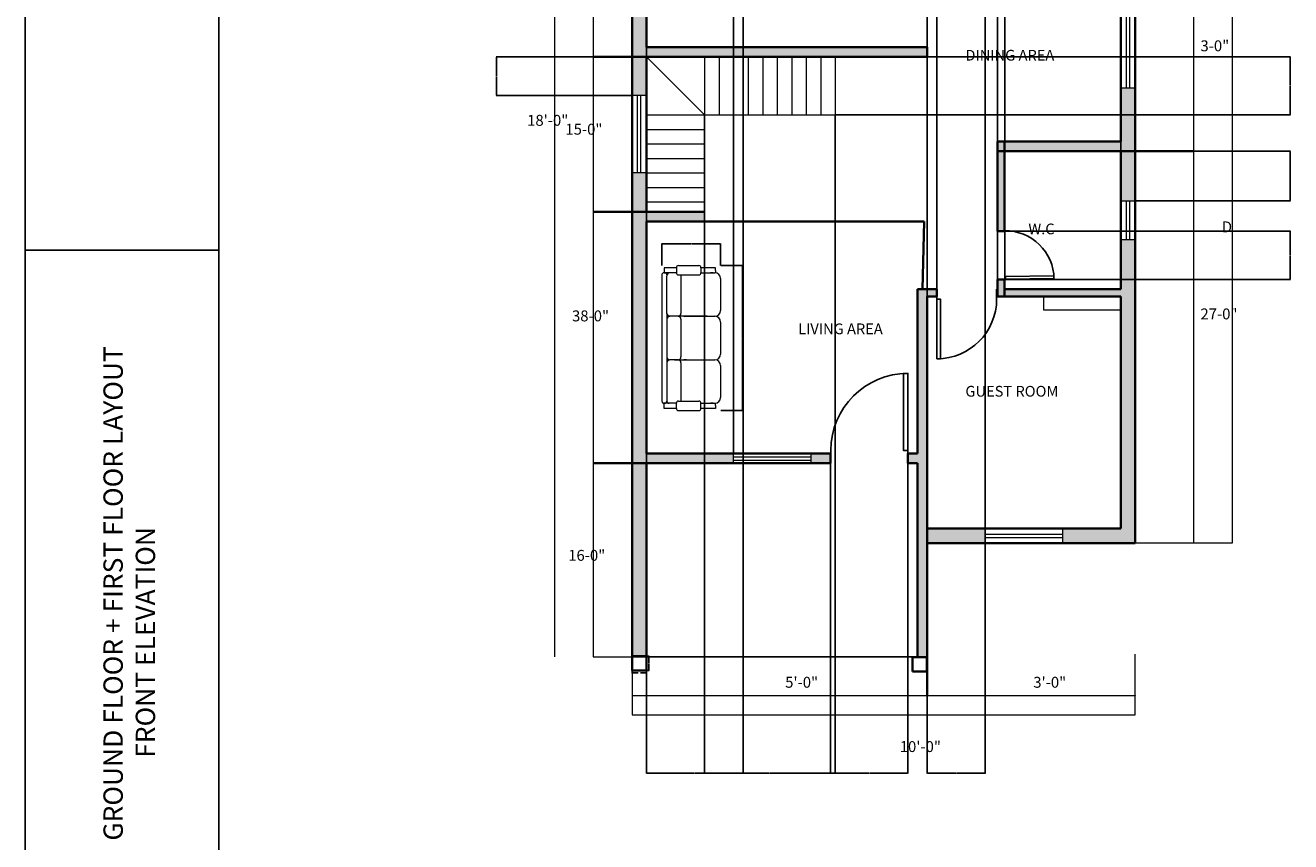
# Model space of a CAD drawing. Units: feet. Extents: x 2813 to 4435, y 1041 to 2557.
# Tile 2 of 6: x 2813 to 3598, y 1649 to 2155. Entities that reach past the tile are written whole.
import ezdxf

# ---------------------------------------------------------------- set-up
doc = ezdxf.new("R2010")
doc.units = ezdxf.units.FT
for name, color, linetype, lineweight in [('A-ANNO-DIMS', 2, 'Continuous', 18), ('A-ANNO-TTLB', 7, 'Continuous', 25), ('A-AREA-IDEN', 7, 'Continuous', 18), ('A-COLS', 7, 'Continuous', 35), ('A-DOOR', 3, 'Continuous', 25), ('A-FLOR', 7, 'Continuous', 25), ('A-FLOR-CASE', 8, 'Continuous', 18), ('A-FLOR-STRS', 7, 'Continuous', 18), ('A-FURN', 8, 'Continuous', 18), ('A-GLAZ', 4, 'Continuous', 18), ('A-WALL', 7, 'Continuous', 35), ('A-WALL-PATT', 252, 'Continuous', 13)]:
    doc.layers.add(name, color=color, linetype=linetype, lineweight=lineweight)
doc.styles.get("Standard").update_dxf_attribs({"font": 'arial.ttf'})
doc.dimstyles.get("Standard").update_dxf_attribs({"dimtxt": 0.18, "dimasz": 0.18, "dimexe": 0.18, "dimexo": 0.0625, "dimgap": 0.09, "dimtad": 0, "dimtih": 1, "dimtoh": 1, "dimdec": 4, "dimzin": 0, "dimdsep": 46, "dimtxsty": 'Standard', "dimcen": 0.09, "dimadec": 0, "dimazin": 0, "dimtfac": 1, "dimtdec": 4, "dimtofl": 0, "dimtmove": 0, "dimatfit": 3, "dimfxl": 1, "dimtolj": 1, "dimtzin": 0, "dimarcsym": 0})

# ---------------------------------------------------------------- blocks, each defined once
blk = doc.blocks.new('F19')
for p, q in [((0.831, 0.019), (-0.909, 0.019)), ((-1.009, -0.011), (-0.939, -0.011)), ((-1.009, -0.181), (-1.009, -0.011)), ((-0.939, -0.181), (-0.939, -0.01)), ((-0.939, -0.011), (-0.939, -0.02)), ((-0.939, -0.177), (-0.939, -0.08)), ((0.213, -0.05), (-0.909, -0.05)), ((-0.298, -0.05), (-0.387, -0.05)), ((-0.339, -0.205), (-0.339, -0.091)), ((-0.339, -0.155), (-0.339, -0.641)), ((0.302, -0.05), (0.213, -0.05)), ((0.261, -0.606), (0.261, -0.051)), ((0.261, -0.205), (0.261, -0.091)), ((0.261, -0.321), (0.261, -0.174)), ((0.301, -0.051), (0.821, -0.051)), ((0.931, -0.011), (0.861, -0.011)), ((0.861, -0.011), (0.861, -0.021)), ((0.861, -0.091), (0.861, -0.011)), ((0.861, -0.181), (0.861, -0.091)), ((0.931, -0.181), (0.931, -0.011)), ((-1.039, -0.211), (-1.039, -0.491)), ((-1.009, -0.181), (-0.939, -0.181)), ((-0.379, -0.245), (-0.911, -0.245)), ((-0.909, -0.211), (-0.909, -0.491)), ((-0.339, -0.321), (-0.339, -0.285)), ((0.221, -0.245), (-0.299, -0.245)), ((0.261, -0.285), (0.261, -0.641)), ((0.829, -0.245), (0.301, -0.245)), ((0.831, -0.211), (0.831, -0.491)), ((0.931, -0.181), (0.861, -0.181)), ((0.961, -0.211), (0.961, -0.491)), ((-1.009, -0.521), (-0.939, -0.521)), ((-1.009, -0.721), (-1.009, -0.521)), ((-0.939, -0.521), (-0.939, -0.691)), ((0.931, -0.521), (0.861, -0.521)), ((0.861, -0.521), (0.861, -0.691)), ((0.931, -0.721), (0.931, -0.521)), ((-0.939, -0.606), (-0.939, -0.711)), ((-0.939, -0.691), (-0.939, -0.65)), ((-0.939, -0.691), (-0.939, -0.711)), ((-0.339, -0.606), (-0.339, -0.711)), ((0.261, -0.606), (0.261, -0.711)), ((0.861, -0.691), (0.861, -0.65)), ((0.861, -0.691), (0.861, -0.711)), ((-0.969, -0.721), (-1.009, -0.721)), ((-0.969, -0.721), (-0.939, -0.721)), ((-0.419, -0.791), (-0.859, -0.791)), ((-0.419, -0.791), (-0.859, -0.791)), ((0.181, -0.791), (-0.259, -0.791)), ((0.027, -0.791), (0.027, -0.791)), ((0.781, -0.791), (0.341, -0.791)), ((0.891, -0.721), (0.86, -0.721)), ((0.891, -0.721), (0.931, -0.721))]:
    blk.add_line(p, q)
for centre, radius, start, end in [((-0.909, -0.011), 0.03, 90, 180), ((0.831, -0.011), 0.03, 360, 90), ((-0.909, -0.02), 0.03, 180, 270), ((-0.909, -0.08), 0.03, 90, 180), ((-0.379, -0.091), 0.04, 0, 90), ((-0.299, -0.091), 0.04, 90, 180), ((0.221, -0.091), 0.04, 0, 90), ((0.301, -0.091), 0.04, 90, 180), ((0.821, -0.091), 0.04, 0, 90), ((0.831, -0.021), 0.03, 270, 360), ((-1.009, -0.211), 0.03, 90, 180), ((-0.939, -0.211), 0.03, 0, 90), ((-0.379, -0.205), 0.04, 270, 360), ((-0.299, -0.205), 0.04, 180, 270), ((0.221, -0.205), 0.04, 270, 360), ((0.301, -0.205), 0.04, 180, 270), ((0.861, -0.211), 0.03, 90, 180), ((0.931, -0.211), 0.03, 0, 90), ((-1.009, -0.491), 0.03, 180, 270), ((-0.939, -0.491), 0.03, 270, 360), ((0.861, -0.491), 0.03, 180, 270), ((0.931, -0.491), 0.03, 270, 360), ((-0.859, -0.711), 0.08, 180, 270), ((-0.419, -0.711), 0.08, 270, 360), ((-0.419, -0.711), 0.08, 270, 360), ((-0.259, -0.711), 0.08, 180, 270), ((0.181, -0.711), 0.08, 270, 360), ((0.341, -0.711), 0.08, 180, 270), ((0.781, -0.711), 0.08, 270, 360)]:
    blk.add_arc(centre, radius, start, end)
blk = doc.blocks.new('A$C5C1B5EFD')
blk.add_blockref('F19', (1.039, 0.791))
blk = doc.blocks.new('*U4')
for p, q in [((0, 0), (0, -5)), ((30, 0), (30, -5))]:
    blk.add_line(p, q)
blk.add_lwpolyline([(0, 0), (0, 30), (1.75, 30), (1.75, 0)], close=True)
blk.add_arc((0, 0), 30, 0, 90)
blk = doc.blocks.new('WINDOW-PLAN-WIDE')
for p, q in [((0, 0), (0, 9)), ((48, 0), (48, 9)), ((0, 5.5), (48, 5.5)), ((0, 3.5), (48, 3.5))]:
    blk.add_line(p, q)
blk = doc.blocks.new('WINDOW-PLAN-NARROW')
for p, q in [((0, 24), (9, 24)), ((3.5, 0), (3.5, 24)), ((5.5, 0), (5.5, 24)), ((0, 0), (9, 0))]:
    blk.add_line(p, q)
blk = doc.blocks.new('WINDOW-PLAN-SLIM-WALL')
for p, q in [((0, 0), (0, 6)), ((0, 4), (48, 4)), ((0, 2), (48, 2)), ((48, 0), (48, 6))]:
    blk.add_line(p, q)
blk = doc.blocks.new('PIER-PLAN-SQUARE')
blk.add_lwpolyline([(0, 0), (9, 0), (9, 9), (0, 9)], close=True)
blk = doc.blocks.new('*D25')
at = {"layer": 'A-ANNO-DIMS', "color": 0, "lineweight": -2, "transparency": 16777216}
for p, q in [((3189.56, 1754.99), (3189.56, 1753.53)), ((3189.74, 1753.71), (3193.28, 1753.71)), ((3198.38, 1753.71), (3194.84, 1753.71)), ((3198.56, 1754.99), (3198.56, 1753.53))]:
    blk.add_line(p, q, dxfattribs=at)
at = {"layer": 'A-ANNO-DIMS', "color": 0, "transparency": 16777216}
for points in [[(3189.74, 1753.74), (3189.74, 1753.68), (3189.56, 1753.71)], [(3198.38, 1753.74), (3198.38, 1753.68), (3198.56, 1753.71)]]:
    blk.add_solid(points, dxfattribs=at)
at = {"layer": 'DEFPOINTS', "color": 0, "transparency": 16777216}
for p in [(3189.56, 1755.06), (3198.56, 1755.06), (3198.56, 1753.71)]:
    blk.add_point(p, dxfattribs=at)
at = {"layer": 'A-ANNO-DIMS', "color": 0, "transparency": 16777216, "insert": (3194.06, 1753.71), "char_height": 0.18, "attachment_point": 5}
blk.add_mtext('\\A1;PIER 9 TYP.', dxfattribs=at)
blk = doc.blocks.new('*D26')
at = {"layer": 'A-ANNO-DIMS', "color": 0, "lineweight": -2, "transparency": 16777216}
for p, q in [((3198.62, 1764.06), (3200.09, 1764.06)), ((3199.91, 1763.88), (3199.91, 1759.74)), ((3199.91, 1755.24), (3199.91, 1759.37)), ((3198.62, 1755.06), (3200.09, 1755.06))]:
    blk.add_line(p, q, dxfattribs=at)
at = {"layer": 'A-ANNO-DIMS', "color": 0, "transparency": 16777216}
for points in [[(3199.88, 1763.88), (3199.94, 1763.88), (3199.91, 1764.06)], [(3199.88, 1755.24), (3199.94, 1755.24), (3199.91, 1755.06)]]:
    blk.add_solid(points, dxfattribs=at)
at = {"layer": 'DEFPOINTS', "color": 0, "transparency": 16777216}
for p in [(3198.56, 1764.06), (3199.91, 1764.06), (3198.56, 1755.06)]:
    blk.add_point(p, dxfattribs=at)
at = {"layer": 'A-ANNO-DIMS', "color": 0, "transparency": 16777216, "insert": (3199.91, 1759.56), "char_height": 0.18, "attachment_point": 5}
blk.add_mtext('\\A1;9 TYP.', dxfattribs=at)
blk = doc.blocks.new('*D33')
at = {"layer": 'A-ANNO-DIMS', "color": 0, "lineweight": -2, "transparency": 16777216}
for p, q in [((3244.52, 2006.2), (3258.13, 2006.2)), ((3257.95, 2006.02), (3257.95, 1961.42)), ((3257.95, 1916.46), (3257.95, 1961.06)), ((3244.52, 1916.28), (3258.13, 1916.28))]:
    blk.add_line(p, q, dxfattribs=at)
at = {"layer": 'A-ANNO-DIMS', "color": 0, "transparency": 16777216}
for points in [[(3257.92, 2006.02), (3257.98, 2006.02), (3257.95, 2006.2)], [(3257.92, 1916.46), (3257.98, 1916.46), (3257.95, 1916.28)]]:
    blk.add_solid(points, dxfattribs=at)
at = {"layer": 'DEFPOINTS', "color": 0, "transparency": 16777216}
for p in [(3244.46, 2006.2), (3257.95, 2006.2), (3244.46, 1916.28)]:
    blk.add_point(p, dxfattribs=at)
at = {"layer": 'A-ANNO-DIMS', "color": 0, "transparency": 16777216, "insert": (3257.95, 1961.24), "char_height": 0.18, "attachment_point": 5}
blk.add_mtext('\\A1;SOFA 90', dxfattribs=at)
blk = doc.blocks.new('*D34')
at = {"layer": 'A-ANNO-DIMS', "color": 0, "lineweight": -2, "transparency": 16777216}
for p, q in [((3208.04, 2006.26), (3208.04, 2019.87)), ((3208.22, 2019.69), (3226.03, 2019.69)), ((3244.28, 2019.69), (3226.47, 2019.69)), ((3244.46, 2006.26), (3244.46, 2019.87))]:
    blk.add_line(p, q, dxfattribs=at)
at = {"layer": 'A-ANNO-DIMS', "color": 0, "transparency": 16777216}
for points in [[(3208.22, 2019.72), (3208.22, 2019.66), (3208.04, 2019.69)], [(3244.28, 2019.72), (3244.28, 2019.66), (3244.46, 2019.69)]]:
    blk.add_solid(points, dxfattribs=at)
at = {"layer": 'DEFPOINTS', "color": 0, "transparency": 16777216}
for p in [(3208.04, 2019.69), (3208.04, 2006.2), (3244.46, 2006.2)]:
    blk.add_point(p, dxfattribs=at)
at = {"layer": 'A-ANNO-DIMS', "color": 0, "transparency": 16777216, "insert": (3226.25, 2019.69), "char_height": 0.18, "attachment_point": 5}
blk.add_mtext('\\A1;36', dxfattribs=at)
blk = doc.blocks.new('*D52')
at = {"layer": 'A-ANNO-DIMS', "color": 0, "lineweight": -2, "transparency": 16777216}
for p, q in [((3198.56, 2333.52), (3198.56, 1691.4)), ((3258.56, 2333.52), (3258.56, 1691.4)), ((3198.74, 1691.58), (3228.34, 1691.58)), ((3258.38, 1691.58), (3228.78, 1691.58))]:
    blk.add_line(p, q, dxfattribs=at)
at = {"layer": 'A-ANNO-DIMS', "color": 0, "transparency": 16777216}
for points in [[(3198.74, 1691.61), (3198.74, 1691.55), (3198.56, 1691.58)], [(3258.38, 1691.61), (3258.38, 1691.55), (3258.56, 1691.58)]]:
    blk.add_solid(points, dxfattribs=at)
at = {"layer": 'DEFPOINTS', "color": 0, "transparency": 16777216}
for p in [(3198.56, 2333.58), (3258.56, 2333.58), (3258.56, 1691.58)]:
    blk.add_point(p, dxfattribs=at)
at = {"layer": 'A-ANNO-DIMS', "color": 0, "transparency": 16777216, "insert": (3228.56, 1691.58), "char_height": 0.18, "attachment_point": 5}
blk.add_mtext('\\A1;60', dxfattribs=at)
blk = doc.blocks.new('*D53')
at = {"layer": 'A-ANNO-DIMS', "color": 0, "lineweight": -2, "transparency": 16777216}
for p, q in [((3372.56, 2333.52), (3372.56, 1691.4)), ((3408.56, 2333.52), (3408.56, 1691.4)), ((3372.74, 1691.58), (3390.34, 1691.58)), ((3408.38, 1691.58), (3390.78, 1691.58))]:
    blk.add_line(p, q, dxfattribs=at)
at = {"layer": 'A-ANNO-DIMS', "color": 0, "transparency": 16777216}
for points in [[(3372.74, 1691.61), (3372.74, 1691.55), (3372.56, 1691.58)], [(3408.38, 1691.61), (3408.38, 1691.55), (3408.56, 1691.58)]]:
    blk.add_solid(points, dxfattribs=at)
at = {"layer": 'DEFPOINTS', "color": 0, "transparency": 16777216}
for p in [(3372.56, 2333.58), (3408.56, 2333.58), (3408.56, 1691.58)]:
    blk.add_point(p, dxfattribs=at)
at = {"layer": 'A-ANNO-DIMS', "color": 0, "transparency": 16777216, "insert": (3390.56, 1691.58), "char_height": 0.18, "attachment_point": 5}
blk.add_mtext('\\A1;36', dxfattribs=at)
blk = doc.blocks.new('*D55')
at = {"layer": 'A-ANNO-DIMS', "color": 0, "lineweight": -2, "transparency": 16777216}
for p, q in [((3315.62, 2135.58), (3597.74, 2135.58)), ((3597.56, 2135.4), (3597.56, 2117.76)), ((3597.56, 2099.76), (3597.56, 2117.4)), ((3315.62, 2099.58), (3597.74, 2099.58))]:
    blk.add_line(p, q, dxfattribs=at)
at = {"layer": 'A-ANNO-DIMS', "color": 0, "transparency": 16777216}
for points in [[(3597.53, 2135.4), (3597.59, 2135.4), (3597.56, 2135.58)], [(3597.53, 2099.76), (3597.59, 2099.76), (3597.56, 2099.58)]]:
    blk.add_solid(points, dxfattribs=at)
at = {"layer": 'DEFPOINTS', "color": 0, "transparency": 16777216}
for p in [(3315.56, 2135.58), (3597.56, 2135.58), (3315.56, 2099.58)]:
    blk.add_point(p, dxfattribs=at)
at = {"layer": 'A-ANNO-DIMS', "color": 0, "transparency": 16777216, "insert": (3597.56, 2117.58), "char_height": 0.18, "attachment_point": 5}
blk.add_mtext('\\A1;36', dxfattribs=at)
blk = doc.blocks.new('*D56')
at = {"layer": 'A-ANNO-DIMS', "color": 0, "lineweight": -2, "transparency": 16777216}
for p, q in [((3234.56, 2099.52), (3234.56, 1691.4)), ((3315.56, 2099.52), (3315.56, 1691.4)), ((3234.74, 1691.58), (3274.86, 1691.58)), ((3315.38, 1691.58), (3275.26, 1691.58))]:
    blk.add_line(p, q, dxfattribs=at)
at = {"layer": 'A-ANNO-DIMS', "color": 0, "transparency": 16777216}
for points in [[(3234.74, 1691.61), (3234.74, 1691.55), (3234.56, 1691.58)], [(3315.38, 1691.61), (3315.38, 1691.55), (3315.56, 1691.58)]]:
    blk.add_solid(points, dxfattribs=at)
at = {"layer": 'DEFPOINTS', "color": 0, "transparency": 16777216}
for p in [(3234.56, 2099.58), (3315.56, 2099.58), (3315.56, 1691.58)]:
    blk.add_point(p, dxfattribs=at)
at = {"layer": 'A-ANNO-DIMS', "color": 0, "transparency": 16777216, "insert": (3275.06, 1691.58), "char_height": 0.18, "attachment_point": 5}
blk.add_mtext('\\A1;81', dxfattribs=at)
blk = doc.blocks.new('*D57')
at = {"layer": 'A-ANNO-DIMS', "color": 0, "lineweight": -2, "transparency": 16777216}
for p, q in [((3198.56, 1889.65), (3198.56, 2414.76)), ((3198.74, 2414.58), (3225.34, 2414.58)), ((3252.38, 2414.58), (3225.78, 2414.58)), ((3252.56, 1889.65), (3252.56, 2414.76))]:
    blk.add_line(p, q, dxfattribs=at)
at = {"layer": 'A-ANNO-DIMS', "color": 0, "transparency": 16777216}
for points in [[(3198.74, 2414.61), (3198.74, 2414.55), (3198.56, 2414.58)], [(3252.38, 2414.61), (3252.38, 2414.55), (3252.56, 2414.58)]]:
    blk.add_solid(points, dxfattribs=at)
at = {"layer": 'DEFPOINTS', "color": 0, "transparency": 16777216}
for p in [(3198.56, 2414.58), (3198.56, 1889.58), (3252.56, 1889.58)]:
    blk.add_point(p, dxfattribs=at)
at = {"layer": 'A-ANNO-DIMS', "color": 0, "transparency": 16777216, "insert": (3225.56, 2414.58), "char_height": 0.18, "attachment_point": 5}
blk.add_mtext('\\A1;54', dxfattribs=at)
blk = doc.blocks.new('*D58')
at = {"layer": 'A-ANNO-DIMS', "color": 0, "lineweight": -2, "transparency": 16777216}
for p, q in [((3312.56, 1883.52), (3312.56, 1691.4)), ((3360.56, 1883.52), (3360.56, 1691.4)), ((3312.74, 1691.58), (3336.33, 1691.58)), ((3360.38, 1691.58), (3336.78, 1691.58))]:
    blk.add_line(p, q, dxfattribs=at)
at = {"layer": 'A-ANNO-DIMS', "color": 0, "transparency": 16777216}
for points in [[(3312.74, 1691.61), (3312.74, 1691.55), (3312.56, 1691.58)], [(3360.38, 1691.61), (3360.38, 1691.55), (3360.56, 1691.58)]]:
    blk.add_solid(points, dxfattribs=at)
at = {"layer": 'DEFPOINTS', "color": 0, "transparency": 16777216}
for p in [(3312.56, 1883.58), (3360.56, 1883.58), (3360.56, 1691.58)]:
    blk.add_point(p, dxfattribs=at)
at = {"layer": 'A-ANNO-DIMS', "color": 0, "transparency": 16777216, "insert": (3336.56, 1691.58), "char_height": 0.18, "attachment_point": 5}
blk.add_mtext('\\A1;48', dxfattribs=at)
blk = doc.blocks.new('*D59')
at = {"layer": 'A-ANNO-DIMS', "color": 0, "lineweight": -2, "transparency": 16777216}
for p, q in [((3420.56, 1991.65), (3420.56, 2414.76)), ((3420.74, 2414.58), (3456.34, 2414.58)), ((3492.38, 2414.58), (3456.77, 2414.58)), ((3492.56, 1991.65), (3492.56, 2414.76))]:
    blk.add_line(p, q, dxfattribs=at)
at = {"layer": 'A-ANNO-DIMS', "color": 0, "transparency": 16777216}
for points in [[(3420.74, 2414.61), (3420.74, 2414.55), (3420.56, 2414.58)], [(3492.38, 2414.61), (3492.38, 2414.55), (3492.56, 2414.58)]]:
    blk.add_solid(points, dxfattribs=at)
at = {"layer": 'DEFPOINTS', "color": 0, "transparency": 16777216}
for p in [(3492.56, 2414.58), (3420.56, 1991.58), (3492.56, 1991.58)]:
    blk.add_point(p, dxfattribs=at)
at = {"layer": 'A-ANNO-DIMS', "color": 0, "transparency": 16777216, "insert": (3456.56, 2414.58), "char_height": 0.18, "attachment_point": 5}
blk.add_mtext('\\A1;72', dxfattribs=at)
blk = doc.blocks.new('*D60')
at = {"layer": 'A-ANNO-DIMS', "color": 0, "lineweight": -2, "transparency": 16777216}
for p, q in [((3372.56, 1834.02), (3372.56, 1691.4)), ((3408.56, 1834.02), (3408.56, 1691.4)), ((3372.74, 1691.58), (3390.34, 1691.58)), ((3408.38, 1691.58), (3390.78, 1691.58))]:
    blk.add_line(p, q, dxfattribs=at)
at = {"layer": 'A-ANNO-DIMS', "color": 0, "transparency": 16777216}
for points in [[(3372.74, 1691.61), (3372.74, 1691.55), (3372.56, 1691.58)], [(3408.38, 1691.61), (3408.38, 1691.55), (3408.56, 1691.58)]]:
    blk.add_solid(points, dxfattribs=at)
at = {"layer": 'DEFPOINTS', "color": 0, "transparency": 16777216}
for p in [(3372.56, 1834.08), (3408.56, 1834.08), (3408.56, 1691.58)]:
    blk.add_point(p, dxfattribs=at)
at = {"layer": 'A-ANNO-DIMS', "color": 0, "transparency": 16777216, "insert": (3390.56, 1691.58), "char_height": 0.18, "attachment_point": 5}
blk.add_mtext('\\A1;36', dxfattribs=at)
blk = doc.blocks.new('*D71')
at = {"layer": 'A-ANNO-DIMS', "color": 0, "lineweight": -2, "transparency": 16777216}
for p, q in [((3420.62, 2027.58), (3597.74, 2027.58)), ((3597.56, 2027.4), (3597.56, 2012.76)), ((3597.56, 1997.76), (3597.56, 2012.4)), ((3420.62, 1997.58), (3597.74, 1997.58))]:
    blk.add_line(p, q, dxfattribs=at)
at = {"layer": 'A-ANNO-DIMS', "color": 0, "transparency": 16777216}
for points in [[(3597.53, 2027.4), (3597.59, 2027.4), (3597.56, 2027.58)], [(3597.53, 1997.76), (3597.59, 1997.76), (3597.56, 1997.58)]]:
    blk.add_solid(points, dxfattribs=at)
at = {"layer": 'DEFPOINTS', "color": 0, "transparency": 16777216}
for p in [(3420.56, 2027.58), (3420.56, 1997.58), (3597.56, 1997.58)]:
    blk.add_point(p, dxfattribs=at)
at = {"layer": 'A-ANNO-DIMS', "color": 0, "transparency": 16777216, "insert": (3597.56, 2012.58), "char_height": 0.18, "attachment_point": 5}
blk.add_mtext('\\A1;30', dxfattribs=at)
blk = doc.blocks.new('*D72')
at = {"layer": 'A-ANNO-DIMS', "color": 0, "lineweight": -2, "transparency": 16777216}
for p, q in [((3378.56, 1991.65), (3378.56, 2414.76)), ((3378.74, 2414.58), (3396.98, 2414.58)), ((3415.88, 2414.58), (3397.63, 2414.58)), ((3416.06, 1987.15), (3416.06, 2414.76))]:
    blk.add_line(p, q, dxfattribs=at)
at = {"layer": 'A-ANNO-DIMS', "color": 0, "transparency": 16777216}
for points in [[(3378.74, 2414.61), (3378.74, 2414.55), (3378.56, 2414.58)], [(3415.88, 2414.61), (3415.88, 2414.55), (3416.06, 2414.58)]]:
    blk.add_solid(points, dxfattribs=at)
at = {"layer": 'DEFPOINTS', "color": 0, "transparency": 16777216}
for p in [(3416.06, 2414.58), (3378.56, 1991.58), (3416.06, 1987.08)]:
    blk.add_point(p, dxfattribs=at)
at = {"layer": 'A-ANNO-DIMS', "color": 0, "transparency": 16777216, "insert": (3397.31, 2414.58), "char_height": 0.18, "attachment_point": 5}
blk.add_mtext('\\A1;37.5', dxfattribs=at)
blk = doc.blocks.new('*D73')
at = {"layer": 'A-ANNO-DIMS', "color": 0, "lineweight": -2, "transparency": 16777216}
for p, q in [((3198.49, 2135.58), (3105.38, 2135.58)), ((3105.56, 2135.4), (3105.56, 2123.76)), ((3105.56, 2111.76), (3105.56, 2123.4)), ((3189.49, 2111.58), (3105.38, 2111.58))]:
    blk.add_line(p, q, dxfattribs=at)
at = {"layer": 'A-ANNO-DIMS', "color": 0, "transparency": 16777216}
for points in [[(3105.53, 2135.4), (3105.59, 2135.4), (3105.56, 2135.58)], [(3105.53, 2111.76), (3105.59, 2111.76), (3105.56, 2111.58)]]:
    blk.add_solid(points, dxfattribs=at)
at = {"layer": 'DEFPOINTS', "color": 0, "transparency": 16777216}
for p in [(3198.56, 2135.58), (3105.56, 2111.58), (3189.56, 2111.58)]:
    blk.add_point(p, dxfattribs=at)
at = {"layer": 'A-ANNO-DIMS', "color": 0, "transparency": 16777216, "insert": (3105.56, 2123.58), "char_height": 0.18, "attachment_point": 5}
blk.add_mtext('\\A1;24', dxfattribs=at)
blk = doc.blocks.new('*D75')
at = {"layer": 'A-ANNO-DIMS', "color": 0, "lineweight": -2, "transparency": 16777216}
for p, q in [((3492.62, 2077.08), (3597.74, 2077.08)), ((3597.56, 2076.9), (3597.56, 2061.89)), ((3597.56, 2046.51), (3597.56, 2061.53)), ((3501.62, 2046.33), (3597.74, 2046.33))]:
    blk.add_line(p, q, dxfattribs=at)
at = {"layer": 'A-ANNO-DIMS', "color": 0, "transparency": 16777216}
for points in [[(3597.53, 2076.9), (3597.59, 2076.9), (3597.56, 2077.08)], [(3597.53, 2046.51), (3597.59, 2046.51), (3597.56, 2046.33)]]:
    blk.add_solid(points, dxfattribs=at)
at = {"layer": 'DEFPOINTS', "color": 0, "transparency": 16777216}
for p in [(3492.56, 2077.08), (3501.56, 2046.33), (3597.56, 2046.33)]:
    blk.add_point(p, dxfattribs=at)
at = {"layer": 'A-ANNO-DIMS', "color": 0, "transparency": 16777216, "insert": (3597.56, 2061.71), "char_height": 0.18, "attachment_point": 5}
blk.add_mtext('\\A1;30.75', dxfattribs=at)

msp = doc.modelspace()

# ---------------------------------------------------------------- hatches: boundary and pattern name
at = {"layer": 'A-WALL-PATT'}
h = msp.add_hatch(color=256, dxfattribs=at)
h.dxf.hatch_style = 1
h.paths.add_polyline_path([(3198.557, 2333.583), (3258.557, 2333.583), (3258.557, 2342.583), (3189.557, 2342.583), (3189.557, 2135.583), (3372.557, 2135.583), (3372.557, 2141.583), (3198.557, 2141.583)])
h.paths.add_polyline_path([(3366.557, 2342.583), (3306.557, 2342.583), (3306.557, 2333.583), (3366.557, 2333.583)], flags=17)
h.paths.add_polyline_path([(3372.557, 2342.583), (3366.557, 2342.583), (3366.557, 2197.083), (3372.557, 2197.083), (3408.557, 2197.083), (3408.557, 2201.583), (3372.557, 2201.583), (3372.557, 2225.773)])
h.paths.add_polyline_path([(3408.557, 2342.583), (3372.557, 2342.583), (3372.557, 2333.583), (3408.557, 2333.583)], flags=17)
h.paths.add_polyline_path([(3501.557, 2342.583), (3456.557, 2342.583), (3456.557, 2333.583), (3492.557, 2333.583), (3492.557, 2201.583), (3456.557, 2201.583), (3456.557, 2197.083), (3501.557, 2197.083)])
h.paths.add_polyline_path([(3501.557, 2197.083), (3492.557, 2197.083), (3492.557, 2164.083), (3501.557, 2164.083)])
h.paths.add_polyline_path([(3501.557, 2116.083), (3492.557, 2116.083), (3492.557, 2083.083), (3420.557, 2083.083), (3420.557, 2077.083), (3501.557, 2077.083)])
h.paths.add_polyline_path([(3501.557, 2077.083), (3492.557, 2077.083), (3492.557, 2046.333), (3501.557, 2046.333)])
h.paths.add_polyline_path([(3501.557, 2022.333), (3492.557, 2022.333), (3492.557, 1991.583), (3420.557, 1991.583), (3420.557, 1987.083), (3492.557, 1987.083), (3492.557, 1843.083), (3456.557, 1843.083), (3456.557, 1834.083), (3501.557, 1834.083)])
h.paths.add_polyline_path([(3408.557, 1843.083), (3372.557, 1843.083), (3372.557, 1834.083), (3408.557, 1834.083)])
h.paths.add_polyline_path([(3372.557, 1987.083), (3378.557, 1987.083), (3378.557, 1991.583), (3372.557, 1991.583), (3366.557, 1991.583), (3366.557, 1889.583), (3360.557, 1889.583), (3360.557, 1883.583), (3366.557, 1883.583), (3366.557, 1763.583), (3372.557, 1763.583)])
h.paths.add_polyline_path([(3198.557, 1883.583), (3189.557, 1883.583), (3189.557, 1763.583), (3198.557, 1763.583)])
h.paths.add_polyline_path([(3198.557, 2033.583), (3234.557, 2033.583), (3234.557, 2039.583), (3189.557, 2039.583), (3189.557, 1883.583), (3198.557, 1883.583), (3252.557, 1883.583), (3252.557, 1889.583), (3198.557, 1889.583)])
h.paths.add_polyline_path([(3198.557, 2063.583), (3189.557, 2063.583), (3189.557, 2039.583), (3198.557, 2039.583)])
h.paths.add_polyline_path([(3198.557, 2135.583), (3189.557, 2135.583), (3189.557, 2111.583), (3198.557, 2111.583)])
h.paths.add_polyline_path([(3312.557, 1889.583), (3300.557, 1889.583), (3300.557, 1883.583), (3312.557, 1883.583)])
h = msp.add_hatch(color=256, dxfattribs=at)
h.dxf.hatch_style = 1
h.paths.add_polyline_path([(3420.557, 1997.583), (3416.057, 1997.583), (3416.057, 1987.083), (3420.557, 1987.083)])
h.paths.add_polyline_path([(3420.557, 2077.083), (3416.057, 2077.083), (3416.057, 2027.583), (3420.557, 2027.583)])
h.paths.add_polyline_path([(3420.557, 2083.083), (3416.057, 2083.083), (3416.057, 2077.083), (3420.557, 2077.083)])

# ---------------------------------------------------------------- linework, layer by layer
at = {"layer": 'A-ANNO-DIMS'}
for p, q in [((3189.557, 2111.583), (3189.557, 2378.583)), ((3141.557, 2342.583), (3141.557, 1763.583)), ((3165.557, 2342.583), (3165.557, 1763.583)), ((3537.557, 2342.583), (3537.557, 1834.083)), ((3561.557, 2342.583), (3561.557, 1834.083)), ((3537.557, 1834.083), (3501.557, 1834.083)), ((3561.557, 1834.083), (3537.557, 1834.083)), ((3501.557, 1727.583), (3501.557, 1765.261)), ((3165.557, 1763.583), (3189.557, 1763.583)), ((3189.557, 1763.583), (3189.557, 1727.583)), ((3189.557, 1739.583), (3501.557, 1739.583)), ((3501.557, 1739.583), (3501.472, 1739.583)), ((3501.557, 1739.583), (3501.501, 1739.529)), ((3501.557, 1739.583), (3501.658, 1739.679)), ((3501.658, 1739.679), (3501.557, 1739.583)), ((3189.557, 1727.583), (3501.557, 1727.583))]:
    msp.add_line(p, q, dxfattribs=at)
at = {"layer": 'A-ANNO-TTLB'}
for p, q in [((2813.466, 1041.465), (2813.466, 2556.562)), ((2933.466, 1041.465), (2933.466, 2556.562)), ((2933.466, 2015.647), (2813.466, 2015.647))]:
    msp.add_line(p, q, dxfattribs=at)
at = {"layer": 'A-FLOR'}
msp.add_line((3189.557, 1763.583), (3372.557, 1763.583), dxfattribs=at)
at = {"layer": 'A-FLOR-CASE'}
msp.add_lwpolyline([(3492.557, 1987.083), (3444.696, 1987.083), (3444.696, 1978.81), (3492.557, 1978.81)], close=True, dxfattribs=at)
at = {"layer": 'A-FLOR-STRS'}
for p, q in [((3234.557, 2099.583), (3198.557, 2135.583)), ((3234.557, 2135.583), (3234.557, 2033.583)), ((3243.557, 2135.583), (3243.557, 2099.583)), ((3252.557, 2135.583), (3252.557, 2099.583)), ((3261.557, 2135.583), (3261.557, 2099.583)), ((3270.557, 2135.583), (3270.557, 2099.583)), ((3279.557, 2135.583), (3279.557, 2099.583)), ((3288.557, 2135.583), (3288.557, 2099.583)), ((3297.557, 2135.583), (3297.557, 2099.583)), ((3306.557, 2135.583), (3306.557, 2099.583)), ((3315.557, 2135.583), (3315.557, 2099.583)), ((3198.557, 2099.583), (3315.557, 2099.583)), ((3198.557, 2090.583), (3234.557, 2090.583)), ((3198.557, 2081.583), (3234.557, 2081.583)), ((3198.557, 2072.583), (3234.557, 2072.583)), ((3198.557, 2063.583), (3234.557, 2063.583)), ((3198.557, 2054.583), (3234.557, 2054.583)), ((3198.557, 2045.583), (3234.557, 2045.583))]:
    msp.add_line(p, q, dxfattribs=at)
at = {"layer": 'A-WALL'}
for p, q in [((3189.557, 2342.583), (3189.557, 1763.583)), ((3501.557, 2342.583), (3501.557, 1834.083)), ((3198.557, 2333.583), (3198.557, 2141.583)), ((3492.557, 2197.083), (3492.557, 2083.083)), ((3198.557, 2141.583), (3372.557, 2141.583)), ((3372.557, 2141.583), (3372.557, 2135.583)), ((3165.557, 2135.583), (3372.557, 2135.583)), ((3198.557, 2135.583), (3198.557, 2039.583)), ((3416.057, 2083.083), (3492.557, 2083.083)), ((3416.057, 2083.083), (3416.057, 2027.583)), ((3420.557, 2083.083), (3420.557, 2027.583)), ((3416.057, 2077.083), (3537.557, 2077.083)), ((3492.557, 2077.083), (3492.557, 1991.583)), ((3165.557, 2039.583), (3234.557, 2039.583)), ((3198.557, 2033.583), (3234.557, 2033.583)), ((3198.557, 2033.583), (3198.557, 1889.583)), ((3234.557, 2033.583), (3370.659, 2033.583)), ((3370.659, 2033.583), (3369.557, 1991.583)), ((3416.057, 2027.583), (3420.557, 2027.583)), ((3416.057, 1997.583), (3420.557, 1997.583)), ((3416.057, 1997.583), (3416.057, 1987.083)), ((3420.557, 1997.583), (3420.557, 1987.083)), ((3366.557, 1991.583), (3372.557, 1991.583)), ((3366.557, 1991.583), (3366.557, 1889.583)), ((3372.557, 1991.583), (3378.557, 1991.583)), ((3372.557, 1987.083), (3372.557, 1739.583)), ((3378.557, 1987.083), (3372.557, 1987.083)), ((3378.557, 1991.583), (3378.557, 1987.083)), ((3416.057, 1987.083), (3492.557, 1987.083)), ((3420.557, 1991.583), (3492.557, 1991.583)), ((3492.557, 1987.083), (3492.557, 1843.083)), ((3165.557, 1883.583), (3312.557, 1883.583)), ((3198.557, 1889.583), (3312.557, 1889.583)), ((3198.557, 1883.583), (3198.557, 1763.583)), ((3312.557, 1883.583), (3312.557, 1889.583)), ((3360.557, 1883.583), (3360.557, 1889.583)), ((3360.557, 1889.583), (3366.557, 1889.583)), ((3360.557, 1883.583), (3366.557, 1883.583)), ((3366.557, 1883.583), (3366.557, 1763.583)), ((3372.557, 1843.083), (3492.557, 1843.083)), ((3372.557, 1834.083), (3501.557, 1834.083))]:
    msp.add_line(p, q, dxfattribs=at)

# ---------------------------------------------------------------- block references
at = {"layer": 'A-COLS'}
for p in [(3189.557, 1755.056), (3363.375, 1754.439)]:
    msp.add_blockref('PIER-PLAN-SQUARE', p, dxfattribs=at)
at = {"layer": 'A-DOOR'}
for p, xscale, yscale, zscale, rotation in [((3421.069, 1997.651), -1.002406396554903, 1.002406396554903, 1.002406396554903, 270.7798030154202), ((3378.557, 1985.411), -1.234420351959542, 1.234420351959542, 1.234420351959542, 180)]:
    msp.add_blockref('*U4', p, dxfattribs=dict(at, xscale=xscale, yscale=yscale, zscale=zscale, rotation=rotation))
at = {"layer": 'A-DOOR', "xscale": -1.592163897733477, "yscale": 1.592163897733477, "zscale": 1.592163897733477}
msp.add_blockref('*U4', (3360.557, 1891.543), dxfattribs=at)
at = {"layer": 'A-FURN', "xscale": 44.96217877560304, "yscale": 44.96217877560304, "zscale": 44.96217877560304, "rotation": 90}
msp.add_blockref('A$C5C1B5EFD', (3244.458, 1916.277), dxfattribs=at)
at = {"layer": 'A-GLAZ'}
for p, rotation in [((3501.557, 2116.083), 90.00000000000063), ((3198.557, 2063.583), 89.9999999999996)]:
    msp.add_blockref('WINDOW-PLAN-WIDE', p, dxfattribs=dict(at, rotation=rotation))
for name, p in [('WINDOW-PLAN-NARROW', (3492.557, 2022.333)), ('WINDOW-PLAN-SLIM-WALL', (3252.557, 1883.583)), ('WINDOW-PLAN-WIDE', (3408.557, 1834.083))]:
    msp.add_blockref(name, p, dxfattribs=at)

# ---------------------------------------------------------------- texts
at = {"layer": 'A-ANNO-DIMS', "char_height": 6.7726, "attachment_point": 1}
for s, insert in [('3-0" ', (3541.928, 2145.786)), ('18\'-0" ', (3124.536, 2099.591)), ('15-0"', (3148.252, 2094.081)), ('D ', (3555.158, 2033.565)), ('38-0" ', (3152.355, 1978.349)), ('27-0"', (3541.928, 1979.573)), ('16-0" ', (3150.007, 1829.936)), ('5\'-0" ', (3284.501, 1751.239)), ('3\'-0" ', (3438.29, 1751.239)), ('10\'-0" ', (3355.525, 1711.366))]:
    msp.add_mtext_dynamic_manual_height_columns(s, width=22.46964, gutter_width=33.863, heights=[0], dxfattribs=dict(at, insert=insert))
at = {"layer": 'A-ANNO-TTLB', "insert": (2861.911, 1649.702), "char_height": 12, "attachment_point": 1, "rotation": 90}
msp.add_mtext_dynamic_manual_height_columns('GROUND FLOOR + FIRST FLOOR LAYOUT\\P              FRONT ELEVATION', width=375.25864, gutter_width=7.02, heights=[0], dxfattribs=at)
at = {"layer": 'A-AREA-IDEN', "attachment_point": 1}
for s, insert, char_height in [('DINING AREA', (3396.207, 2139.888), 6.65198), ('W.C', (3435.241, 2032.197), 6.652), ('LIVING AREA', (3292.532, 1970.265), 6.65198), ('GUEST ROOM', (3396.207, 1931.578), 6.652)]:
    msp.add_mtext_dynamic_manual_height_columns(s, width=109.65837, gutter_width=33.26, heights=[0], dxfattribs=dict(at, insert=insert, char_height=char_height))

# ---------------------------------------------------------------- dimensions: what is measured, and where the dimension line sits
at = {"layer": 'A-ANNO-DIMS'}
for base, p1, p2, override, picture, middle in [((3198.557, 2414.583), (3252.557, 1889.583), (3198.557, 1889.583), {"dimdec": 0, "dimlfac": 1, "dimrnd": 0, "dimzin": 0, "dimdsep": 46, "dimlunit": 2}, '*D57', (3225.557, 2414.583)), ((3416.057, 2414.583), (3378.557, 1991.583), (3416.057, 1987.083), {"dimdec": 1, "dimlfac": 1, "dimrnd": 0, "dimzin": 0, "dimdsep": 46, "dimlunit": 2}, '*D72', (3397.307, 2414.583)), ((3492.557, 2414.583), (3420.557, 1991.583), (3492.557, 1991.583), {"dimdec": 0, "dimlfac": 1, "dimrnd": 0, "dimzin": 0, "dimdsep": 46, "dimlunit": 2}, '*D59', (3456.557, 2414.583)), ((3258.557, 1691.583), (3198.557, 2333.583), (3258.557, 2333.583), {"dimdec": 0, "dimlfac": 1, "dimrnd": 0, "dimzin": 0, "dimdsep": 46, "dimlunit": 2}, '*D52', (3228.557, 1691.583)), ((3408.557, 1691.583), (3372.557, 2333.583), (3408.557, 2333.583), {"dimdec": 0, "dimlfac": 1, "dimrnd": 0, "dimzin": 0, "dimdsep": 46, "dimlunit": 2}, '*D53', (3390.557, 1691.583)), ((3315.557, 1691.583), (3234.557, 2099.583), (3315.557, 2099.583), {"dimdec": 0, "dimlfac": 1, "dimrnd": 0, "dimzin": 0, "dimdsep": 46, "dimlunit": 2}, '*D56', (3275.057, 1691.583)), ((3360.557, 1691.583), (3312.557, 1883.583), (3360.557, 1883.583), {"dimdec": 0, "dimlfac": 1, "dimrnd": 0, "dimzin": 0, "dimdsep": 46, "dimlunit": 2}, '*D58', (3336.557, 1691.583)), ((3408.557, 1691.583), (3372.557, 1834.083), (3408.557, 1834.083), {"dimdec": 0, "dimlfac": 1, "dimrnd": 0, "dimzin": 0, "dimdsep": 46, "dimlunit": 2}, '*D60', (3390.557, 1691.583))]:
    dim = msp.add_linear_dim(base=base, p1=p1, p2=p2, dimstyle='Standard', override=override, dxfattribs=at)
    dim.commit()
    dim.dimension.update_dxf_attribs({"geometry": picture, "text_midpoint": middle})
for base, p1, p2, angle, override, picture, middle in [((3105.557, 2111.583), (3198.557, 2135.583), (3189.557, 2111.583), 90, {"dimdec": 0, "dimlfac": 1, "dimrnd": 0, "dimzin": 0, "dimdsep": 46, "dimlunit": 2}, '*D73', (3105.557, 2123.583)), ((3597.557, 2135.583), (3315.557, 2099.583), (3315.557, 2135.583), 90, {"dimdec": 0, "dimlfac": 1, "dimrnd": 0, "dimzin": 0, "dimdsep": 46, "dimlunit": 2}, '*D55', (3597.557, 2117.583)), ((3597.557, 2046.333), (3492.557, 2077.083), (3501.557, 2046.333), 90, {"dimdec": 2, "dimlfac": 1, "dimrnd": 0, "dimzin": 0, "dimdsep": 46, "dimlunit": 2}, '*D75', (3597.557, 2061.708)), ((3597.557, 1997.583), (3420.557, 2027.583), (3420.557, 1997.583), 90, {"dimdec": 0, "dimlfac": 1, "dimrnd": 0, "dimzin": 0, "dimdsep": 46, "dimlunit": 2}, '*D71', (3597.557, 2012.583)), ((3208.039, 2019.69), (3244.458, 2006.201), (3208.039, 2006.201), 180, {"dimdec": 0, "dimlfac": 1, "dimrnd": 0, "dimzin": 0, "dimdsep": 46, "dimlunit": 2}, '*D34', (3226.248, 2019.69))]:
    dim = msp.add_linear_dim(base=base, p1=p1, p2=p2, angle=angle, dimstyle='Standard', override=override, dxfattribs=at)
    dim.commit()
    dim.dimension.update_dxf_attribs({"geometry": picture, "text_midpoint": middle})
for base, p1, p2, text, picture, middle in [((3257.947, 2006.201), (3244.458, 1916.277), (3244.458, 2006.201), 'SOFA <>', '*D33', (3257.947, 1961.239)), ((3199.907, 1764.056), (3198.557, 1755.056), (3198.557, 1764.056), '<> TYP.', '*D26', (3199.907, 1759.556))]:
    dim = msp.add_linear_dim(base=base, p1=p1, p2=p2, angle=90, text=text, dimstyle='Standard', override={"dimdec": 0, "dimlfac": 1, "dimrnd": 0, "dimzin": 0, "dimdsep": 46, "dimlunit": 2}, dxfattribs=at)
    dim.commit()
    dim.dimension.update_dxf_attribs({"geometry": picture, "text_midpoint": middle})
dim = msp.add_linear_dim(base=(3198.557, 1753.706), p1=(3189.557, 1755.056), p2=(3198.557, 1755.056), text='PIER <> TYP.', dimstyle='Standard', override={"dimdec": 0, "dimlfac": 1, "dimrnd": 0, "dimzin": 0, "dimdsep": 46, "dimlunit": 2}, dxfattribs=at)
dim.commit()
dim.dimension.update_dxf_attribs({"geometry": '*D25', "text_midpoint": (3194.057, 1753.706)})

doc.saveas('drawing.dxf')
